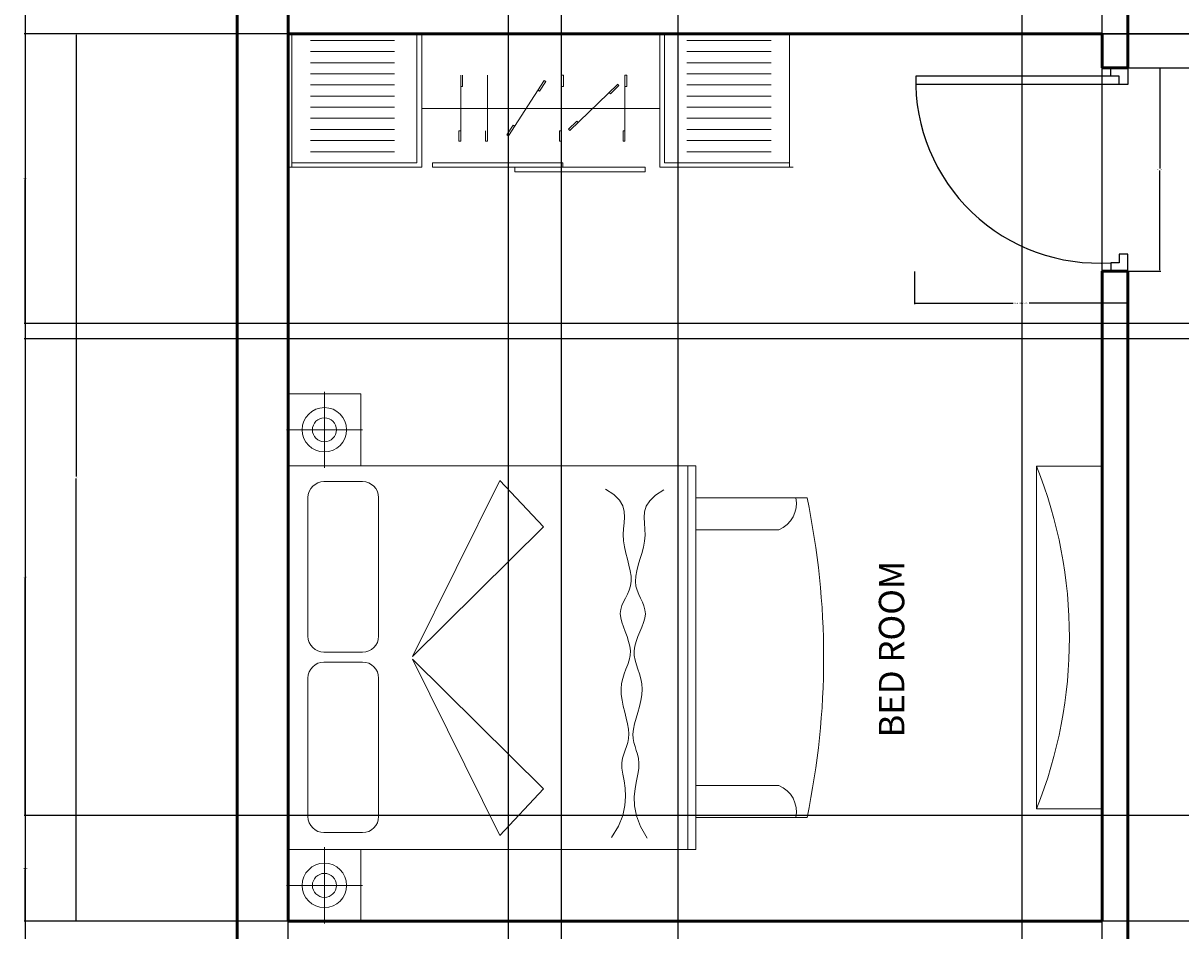
# Model space of a CAD drawing. Units: inches. Extents: x 1865 to 2541, y 1997 to 2759.
# Tile 6 of 11: x 1865 to 2070, y 2405 to 2566. Entities that reach past the tile are written whole.
import ezdxf

# ---------------------------------------------------------------- set-up
doc = ezdxf.new("R2010")
doc.units = ezdxf.units.IN
for name, color, linetype, lineweight in [('A-ANNO-DIMS', 2, 'Continuous', 18), ('A-AREA-IDEN', 4, 'Continuous', 18), ('A-WALL', 7, 'Continuous', 50), ('BED', 42, 'Continuous', 13), ('CUPBOARD', 61, 'Continuous', 18), ('DOOR', 1, 'Continuous', 25), ('TV', 3, 'Continuous', 18)]:
    doc.layers.add(name, color=color, linetype=linetype, lineweight=lineweight)
doc.styles.get("Standard").update_dxf_attribs({"font": 'arial.ttf'})
doc.dimstyles.get("Standard").update_dxf_attribs({"dimtxt": 0.18, "dimasz": 0.18, "dimexe": 0.18, "dimexo": 0.0625, "dimgap": 0.09, "dimtad": 0, "dimtih": 1, "dimtoh": 1, "dimdec": 4, "dimzin": 0, "dimdsep": 46, "dimtxsty": 'Standard', "dimcen": 0.09, "dimadec": 0, "dimazin": 0, "dimtfac": 1, "dimtdec": 4, "dimtofl": 0, "dimtmove": 0, "dimatfit": 3, "dimfxl": 1, "dimtolj": 1, "dimtzin": 0, "dimarcsym": 0})

# ---------------------------------------------------------------- blocks, each defined once
blk = doc.blocks.new('A$C4F543DC7')
for p, q in [((0.0134, 3.35, -0.1688), (3.3134, 3.35, -0.1688)), ((0.4634, 3.35, -0.1688), (0.0134, 3.35, -0.1688)), ((0.0134, 2.896, -0.1688), (0.0134, 3.35, -0.1688)), ((0.0134, 3.35, -0.1688), (0.0134, 2.896, -0.1688)), ((0.2381, 3.1233, -0.4388), (0.2381, 3.3614, -0.4388)), ((0.4634, 3.35, -0.1688), (0.4634, 0.8, -0.1688)), ((2.8634, 3.35, -0.1688), (0.4634, 3.35, -0.1688)), ((0.4634, 2.896, -0.1688), (0.4634, 3.35, -0.1688)), ((2.8634, 0.8, -0.1688), (2.8634, 3.35, -0.1688)), ((2.8634, 3.35, -0.1688), (3.3134, 3.35, -0.1688)), ((2.8634, 2.896, -0.1688), (2.8634, 3.35, -0.1688)), ((3.0888, 3.1233, -0.4388), (3.0888, 3.3614, -0.4388)), ((3.3134, 3.35, -0.1688), (3.3134, 2.896, -0.1688)), ((3.3134, 3.35, -0.1688), (3.3134, 2.896, -0.1688)), ((1.5354, 3.226, -0.1688), (0.6684, 3.226, -0.1688)), ((2.6644, 3.226, -0.1688), (1.7974, 3.226, -0.1688)), ((0.2381, 3.1233, -0.4388), (0, 3.1233, -0.4388)), ((0.2381, 3.1233, -0.4388), (0.4762, 3.1233, -0.4388)), ((0.2381, 3.1233, -0.4388), (0.2381, 2.8852, -0.4388)), ((0.5684, 3.126, -0.1688), (0.5684, 2.884, -0.1688)), ((1.6354, 2.884, -0.1688), (1.6354, 3.126, -0.1688)), ((1.6974, 3.126, -0.1688), (1.6974, 2.884, -0.1688)), ((2.7644, 2.884, -0.1688), (2.7644, 3.126, -0.1688)), ((3.0888, 3.1233, -0.4388), (2.8507, 3.1233, -0.4388)), ((3.0888, 3.1233, -0.4388), (3.0888, 2.8852, -0.4388)), ((3.0888, 3.1233, -0.4388), (3.3269, 3.1233, -0.4388)), ((0.4634, 2.896, -0.1688), (0.0134, 2.896, -0.1688)), ((0.0134, 2.896, -0.1688), (0.4634, 2.896, -0.1688)), ((0.4634, 0.8, -0.1688), (0.4634, 2.896, -0.1688)), ((2.8634, 2.896, -0.1688), (2.8634, 0.8, -0.1688)), ((3.3134, 2.896, -0.1688), (2.8634, 2.896, -0.1688)), ((3.3134, 2.896, -0.1688), (2.8634, 2.896, -0.1688)), ((0.6684, 2.784, -0.1688), (1.5354, 2.784, -0.1688)), ((1.7974, 2.784, -0.1688), (2.6644, 2.784, -0.1688)), ((1.6534, 2.573, -0.1688), (0.5504, 2.025, -0.1688)), ((0.8414, 1.752, -0.1688), (1.6534, 2.573, -0.1688)), ((2.4814, 1.752, -0.1688), (1.6694, 2.573, -0.1688)), ((1.6694, 2.573, -0.1688), (2.7724, 2.025, -0.1688)), ((0.5504, 2.025, -0.1688), (0.8414, 1.752, -0.1688)), ((2.7724, 2.025, -0.1688), (2.4814, 1.752, -0.1688)), ((0.5369, 1.3267, -0.1688), (0.6088, 1.2835, -0.1688)), ((2.6479, 1.2774, -0.1688), (2.683, 1.312, -0.1688)), ((2.683, 1.312, -0.1688), (2.7182, 1.3641, -0.1688)), ((0.6088, 1.2835, -0.1688), (0.6756, 1.2566, -0.1688)), ((0.6756, 1.2566, -0.1688), (0.7373, 1.2428, -0.1688)), ((0.7373, 1.2428, -0.1688), (0.794, 1.239, -0.1688)), ((0.794, 1.239, -0.1688), (0.8457, 1.242, -0.1688)), ((0.8457, 1.242, -0.1688), (0.8925, 1.2489, -0.1688)), ((0.8925, 1.2489, -0.1688), (0.9345, 1.2564, -0.1688)), ((0.9345, 1.2564, -0.1688), (0.9718, 1.2615, -0.1688)), ((0.9718, 1.2615, -0.1688), (1.0044, 1.2617, -0.1688)), ((1.0044, 1.2617, -0.1688), (1.0334, 1.2578, -0.1688)), ((1.0334, 1.2578, -0.1688), (1.0597, 1.2509, -0.1688)), ((1.0597, 1.2509, -0.1688), (1.0842, 1.2424, -0.1688)), ((1.0842, 1.2424, -0.1688), (1.1081, 1.2336, -0.1688)), ((1.1081, 1.2336, -0.1688), (1.1322, 1.2257, -0.1688)), ((1.2498, 1.2264, -0.1688), (1.2852, 1.2347, -0.1688)), ((1.2852, 1.2347, -0.1688), (1.3218, 1.2441, -0.1688)), ((1.3218, 1.2441, -0.1688), (1.3591, 1.2533, -0.1688)), ((1.3591, 1.2533, -0.1688), (1.3963, 1.2612, -0.1688)), ((1.3963, 1.2612, -0.1688), (1.4328, 1.2664, -0.1688)), ((1.4328, 1.2664, -0.1688), (1.4679, 1.2677, -0.1688)), ((1.4679, 1.2677, -0.1688), (1.501, 1.2643, -0.1688)), ((1.501, 1.2643, -0.1688), (1.5324, 1.257, -0.1688)), ((1.5324, 1.257, -0.1688), (1.5624, 1.2473, -0.1688)), ((1.5624, 1.2473, -0.1688), (1.5915, 1.2365, -0.1688)), ((1.5915, 1.2365, -0.1688), (1.6199, 1.2259, -0.1688)), ((1.7955, 1.2301, -0.1688), (1.8258, 1.2417, -0.1688)), ((1.8258, 1.2417, -0.1688), (1.8557, 1.2531, -0.1688)), ((1.8557, 1.2531, -0.1688), (1.8849, 1.263, -0.1688)), ((1.8849, 1.263, -0.1688), (1.913, 1.2698, -0.1688)), ((1.913, 1.2698, -0.1688), (1.9397, 1.2722, -0.1688)), ((1.9397, 1.2722, -0.1688), (1.9649, 1.2692, -0.1688)), ((1.9649, 1.2692, -0.1688), (1.989, 1.2617, -0.1688)), ((1.989, 1.2617, -0.1688), (2.0124, 1.2512, -0.1688)), ((2.0124, 1.2512, -0.1688), (2.0359, 1.2391, -0.1688)), ((2.0359, 1.2391, -0.1688), (2.0599, 1.2269, -0.1688)), ((2.2791, 1.2279, -0.1688), (2.3173, 1.2378, -0.1688)), ((2.3173, 1.2378, -0.1688), (2.3558, 1.2465, -0.1688)), ((2.3558, 1.2465, -0.1688), (2.3944, 1.2527, -0.1688)), ((2.3944, 1.2527, -0.1688), (2.4325, 1.255, -0.1688)), ((2.4325, 1.255, -0.1688), (2.4698, 1.2529, -0.1688)), ((2.4698, 1.2529, -0.1688), (2.5064, 1.2488, -0.1688)), ((2.5064, 1.2488, -0.1688), (2.5423, 1.2459, -0.1688)), ((2.5423, 1.2459, -0.1688), (2.5777, 1.2476, -0.1688)), ((2.5777, 1.2476, -0.1688), (2.6129, 1.257, -0.1688)), ((2.6129, 1.257, -0.1688), (2.6479, 1.2774, -0.1688)), ((0.6067, 1.1458, -0.1688), (0.6743, 1.1706, -0.1688)), ((0.6743, 1.1706, -0.1688), (0.7364, 1.1825, -0.1688)), ((0.7364, 1.1825, -0.1688), (0.7931, 1.1846, -0.1688)), ((0.7931, 1.1846, -0.1688), (0.8447, 1.1799, -0.1688)), ((0.8447, 1.1799, -0.1688), (0.8913, 1.1716, -0.1688)), ((0.8913, 1.1716, -0.1688), (0.9331, 1.1628, -0.1688)), ((0.9331, 1.1628, -0.1688), (0.9701, 1.1565, -0.1688)), ((1.0318, 1.1582, -0.1688), (1.0583, 1.1642, -0.1688)), ((1.0583, 1.1642, -0.1688), (1.0831, 1.172, -0.1688)), ((1.0831, 1.172, -0.1688), (1.1072, 1.18, -0.1688)), ((1.1072, 1.18, -0.1688), (1.1316, 1.1872, -0.1688)), ((1.1316, 1.1872, -0.1688), (1.1573, 1.192, -0.1688)), ((1.1322, 1.2257, -0.1688), (1.1577, 1.2201, -0.1688)), ((1.1573, 1.192, -0.1688), (1.1851, 1.1932, -0.1688)), ((1.1577, 1.2201, -0.1688), (1.1855, 1.218, -0.1688)), ((1.1851, 1.1932, -0.1688), (1.2158, 1.1898, -0.1688)), ((1.1855, 1.218, -0.1688), (1.2163, 1.2204, -0.1688)), ((1.2158, 1.1898, -0.1688), (1.2491, 1.1828, -0.1688)), ((1.2163, 1.2204, -0.1688), (1.2498, 1.2264, -0.1688)), ((1.2491, 1.1828, -0.1688), (1.2842, 1.1734, -0.1688)), ((1.2842, 1.1734, -0.1688), (1.3206, 1.1629, -0.1688)), ((1.3206, 1.1629, -0.1688), (1.3575, 1.1524, -0.1688)), ((1.5609, 1.152, -0.1688), (1.5903, 1.1619, -0.1688)), ((1.5903, 1.1619, -0.1688), (1.6191, 1.1716, -0.1688)), ((1.6191, 1.1716, -0.1688), (1.6475, 1.1797, -0.1688)), ((1.6199, 1.2259, -0.1688), (1.6481, 1.2169, -0.1688)), ((1.6475, 1.1797, -0.1688), (1.676, 1.1849, -0.1688)), ((1.6481, 1.2169, -0.1688), (1.6765, 1.2108, -0.1688)), ((1.676, 1.1849, -0.1688), (1.7049, 1.1858, -0.1688)), ((1.6765, 1.2108, -0.1688), (1.7053, 1.209, -0.1688)), ((1.7049, 1.1858, -0.1688), (1.7344, 1.1816, -0.1688)), ((1.7053, 1.209, -0.1688), (1.7349, 1.2124, -0.1688)), ((1.7344, 1.1816, -0.1688), (1.7643, 1.1731, -0.1688)), ((1.7349, 1.2124, -0.1688), (1.7651, 1.2199, -0.1688)), ((1.7643, 1.1731, -0.1688), (1.7944, 1.1619, -0.1688)), ((1.7651, 1.2199, -0.1688), (1.7955, 1.2301, -0.1688)), ((1.7944, 1.1619, -0.1688), (1.8244, 1.1494, -0.1688)), ((2.0588, 1.1568, -0.1688), (2.0842, 1.167, -0.1688)), ((2.0599, 1.2269, -0.1688), (2.0849, 1.216, -0.1688)), ((2.0842, 1.167, -0.1688), (2.1112, 1.1743, -0.1688)), ((2.0849, 1.216, -0.1688), (2.1117, 1.2077, -0.1688)), ((2.1112, 1.1743, -0.1688), (2.1403, 1.1775, -0.1688)), ((2.1117, 1.2077, -0.1688), (2.1407, 1.2037, -0.1688)), ((2.1403, 1.1775, -0.1688), (2.1718, 1.1755, -0.1688)), ((2.1407, 1.2037, -0.1688), (2.1723, 1.2047, -0.1688)), ((2.1718, 1.1755, -0.1688), (2.2056, 1.1691, -0.1688)), ((2.1723, 1.2047, -0.1688), (2.2062, 1.21, -0.1688)), ((2.2056, 1.1691, -0.1688), (2.2411, 1.1598, -0.1688)), ((2.2062, 1.21, -0.1688), (2.242, 1.2182, -0.1688)), ((2.2411, 1.1598, -0.1688), (2.2779, 1.1489, -0.1688)), ((2.242, 1.2182, -0.1688), (2.2791, 1.2279, -0.1688)), ((0.5334, 1.105, -0.1688), (0.6067, 1.1458, -0.1688)), ((0.9701, 1.1565, -0.1688), (1.0027, 1.1552, -0.1688)), ((1.0027, 1.1552, -0.1688), (1.0318, 1.1582, -0.1688)), ((1.3575, 1.1524, -0.1688), (1.3945, 1.1434, -0.1688)), ((1.3945, 1.1434, -0.1688), (1.4308, 1.1371, -0.1688)), ((1.4308, 1.1371, -0.1688), (1.4658, 1.1347, -0.1688)), ((1.4658, 1.1347, -0.1688), (1.499, 1.137, -0.1688)), ((1.499, 1.137, -0.1688), (1.5306, 1.1433, -0.1688)), ((1.5306, 1.1433, -0.1688), (1.5609, 1.152, -0.1688)), ((1.8244, 1.1494, -0.1688), (1.8539, 1.137, -0.1688)), ((1.8539, 1.137, -0.1688), (1.8827, 1.1263, -0.1688)), ((1.8827, 1.1263, -0.1688), (1.9106, 1.1186, -0.1688)), ((1.9106, 1.1186, -0.1688), (1.9373, 1.1153, -0.1688)), ((1.9373, 1.1153, -0.1688), (1.9625, 1.1176, -0.1688)), ((1.9625, 1.1176, -0.1688), (1.9868, 1.1243, -0.1688)), ((1.9868, 1.1243, -0.1688), (2.0106, 1.134, -0.1688)), ((2.0106, 1.134, -0.1688), (2.0344, 1.1454, -0.1688)), ((2.0344, 1.1454, -0.1688), (2.0588, 1.1568, -0.1688)), ((2.2779, 1.1489, -0.1688), (2.3157, 1.1379, -0.1688)), ((2.3157, 1.1379, -0.1688), (2.354, 1.1279, -0.1688)), ((2.354, 1.1279, -0.1688), (2.3923, 1.1205, -0.1688)), ((2.3923, 1.1205, -0.1688), (2.4304, 1.117, -0.1688)), ((2.4304, 1.117, -0.1688), (2.4677, 1.118, -0.1688)), ((2.4677, 1.118, -0.1688), (2.5043, 1.1209, -0.1688)), ((2.5043, 1.1209, -0.1688), (2.5403, 1.1226, -0.1688)), ((2.5403, 1.1226, -0.1688), (2.5757, 1.1199, -0.1688)), ((2.5757, 1.1199, -0.1688), (2.6106, 1.1094, -0.1688)), ((2.6106, 1.1094, -0.1688), (2.645, 1.0879, -0.1688)), ((2.645, 1.0879, -0.1688), (2.6789, 1.0522, -0.1688)), ((2.6789, 1.0522, -0.1688), (2.7124, 0.999, -0.1688)), ((0.4634, 0.85, -0.1688), (2.8634, 0.85, -0.1688)), ((0.4634, 0.8, -0.1688), (2.8634, 0.8, -0.1688)), ((0.6634, 0.8, -0.1688), (0.4634, 0.8, -0.1688)), ((0.6634, 0.8, -0.1688), (2.6634, 0.8, -0.1688)), ((0.6634, 0.104, -0.1688), (0.6634, 0.8, -0.1688)), ((0.6634, 0.104, -0.1688), (0.6634, 0.8, -0.1688)), ((0.8634, 0.281, -0.1688), (0.8634, 0.8, -0.1688)), ((2.4634, 0.8, -0.1688), (2.4634, 0.281, -0.1688)), ((2.8634, 0.8, -0.1688), (2.6634, 0.8, -0.1688)), ((2.6634, 0.8, -0.1688), (2.6634, 0.104, -0.1688)), ((2.6634, 0.8, -0.1688), (2.6634, 0.104, -0.1688))]:
    blk.add_line(p, q)
for centre, radius in [((0.2381, 3.1233, -0.4388), 0.139), ((3.0888, 3.1233, -0.4388), 0.139), ((0.2381, 3.1233, -0.4388), 0.075), ((3.0888, 3.1233, -0.4388), 0.075)]:
    blk.add_circle(centre, radius)
for centre, radius, start, end in [((0.6684, 3.126, -0.1688), 0.1, 90, 180), ((1.5354, 3.126, -0.1688), 0.1, 0, 90), ((1.7974, 3.126, -0.1688), 0.1, 90, 180), ((2.6644, 3.126, -0.1688), 0.1, 0, 90), ((0.6684, 2.884, -0.1688), 0.1, 180, 270), ((1.5354, 2.884, -0.1688), 0.1, 270, 0), ((1.7974, 2.884, -0.1688), 0.1, 180, 270), ((2.6644, 2.884, -0.1688), 0.1, 270, 0), ((0.6994, 0.3472, -0.1688), 0.1769, 258.2616, 338.03196), ((2.6275, 0.3472, -0.1688), 0.1769, 201.96804, 281.7384), ((1.6634, 4.8597, -0.1688), 4.8597, 258.12517, 281.87483), ((1.6634, 4.8597, -0.1688), 4.8597, 258.12517, 281.87483)]:
    blk.add_arc(centre, radius, start, end)
blk = doc.blocks.new('A$C34930FF8')
at = {"ltscale": 0.05}
for p, q in [((0, 2252.4), (0, 16.8)), ((600, 2252.4), (0, 2252.4)), ((185.4, 1513), (185.4, 1521.5)), ((237.7, 1513), (237.7, 1521.5)), ((436.7, 1513), (436.7, 1504.4)), ((482.5, 1513), (482.5, 1504.4)), ((227.1, 1479.2), (233.2, 1485.2)), ((263.6, 1441.7), (269.7, 1447.7)), ((398.2, 1303.6), (392.1, 1297.6)), ((434.8, 1266.1), (428.7, 1260.1)), ((185.4, 1229.1), (185.4, 1237.7)), ((237.7, 1229.1), (237.7, 1237.7)), ((436.7, 1228.2), (436.7, 1219.7)), ((482.5, 1228.2), (482.5, 1219.7)), ((209.5, 1150.1), (214.1, 1157.3)), ((253.5, 1121.8), (258.1, 1129)), ((415.3, 1017.6), (410.6, 1010.5)), ((459.3, 989.3), (454.7, 982.1)), ((482.5, 894.9), (482.5, 886.3)), ((237.7, 775.3), (237.7, 783.9)), ((436.7, 775.3), (436.7, 766.8)), ((482.5, 775.3), (482.5, 766.8)), ((600, 16.8), (0, 16.8))]:
    blk.add_line(p, q, dxfattribs=at)
for p, q in [((580, 1690.9), (580, 2252.4)), ((600, 1669.3), (600, 2269.3)), ((30, 1790.9), (30, 2169.3)), ((80, 1790.9), (80, 2169.3)), ((130, 1790.9), (130, 2169.3)), ((180, 1790.9), (180, 2169.3)), ((230, 1790.9), (230, 2169.3)), ((280, 1790.9), (280, 2169.3)), ((330, 1790.9), (330, 2169.3)), ((380, 1790.9), (380, 2169.3)), ((430, 1790.9), (430, 2169.3)), ((480, 1790.9), (480, 2169.3)), ((530, 1790.9), (530, 2169.3)), ((580, 1690.9), (0, 1690.9)), ((600, 1669.3), (0, 1669.3)), ((335.4, 1666.1), (335.4, 603.1)), ((600, 1603.3), (620, 1603.3)), ((600, 1018.7), (600, 1603.3)), ((620, 1603.3), (620, 1018.7)), ((237.7, 1521.5), (185.4, 1521.5)), ((482.5, 1513), (185.4, 1513)), ((434.8, 1266.1), (227.4, 1478.9)), ((269.7, 1447.7), (233.2, 1485.2)), ((436.7, 1504.4), (482.5, 1504.4)), ((428.7, 1260.1), (392.1, 1297.6)), ((237.7, 1237.7), (185.4, 1237.7)), ((482.5, 1228.2), (185.4, 1228.2)), ((436.7, 1219.7), (482.5, 1219.7)), ((600, 1233.4), (580, 1233.4)), ((580, 1233.4), (580, 648.7)), ((600, 648.7), (600, 1233.4)), ((459.3, 989.3), (209.5, 1150.1)), ((258.1, 1129), (214.1, 1157.3)), ((454.7, 982.1), (410.6, 1010.5)), ((620, 1018.7), (600, 1018.7)), ((482.5, 894.9), (185.4, 894.9)), ((436.7, 886.3), (482.5, 886.3)), ((237.7, 783.9), (185.4, 783.9)), ((482.5, 775.3), (185.4, 775.3)), ((436.7, 766.8), (482.5, 766.8)), ((580, 648.7), (600, 648.7)), ((600, 600), (0, 600)), ((580, 578.3), (0, 578.3)), ((580, 578.3), (580, 16.8)), ((600, 600), (600, 0)), ((30, 478.3), (30, 100)), ((80, 478.3), (80, 100)), ((130, 478.3), (130, 100)), ((180, 478.3), (180, 100)), ((230, 478.3), (230, 100)), ((280, 478.3), (280, 100)), ((330, 478.3), (330, 100)), ((380, 478.3), (380, 100)), ((430, 478.3), (430, 100)), ((480, 478.3), (480, 100)), ((530, 478.3), (530, 100))]:
    blk.add_line(p, q)
blk = doc.blocks.new('DOOR-SWING-36IN')
for p, q in [((34.51, 36), (37.51, 36)), ((34.51, 34.5), (34.51, 36)), ((37.51, 36), (37.51, 33)), ((36.01, 34.5), (0.01, 34.5)), ((36.01, 33), (0.01, 33)), ((36.01, 34.5), (34.51, 34.5)), ((36.01, 33), (36.01, 34.5)), ((37.51, 33), (36.01, 33)), ((37.51, 3), (36.01, 3)), ((36.01, 3), (36.01, 1.5)), ((37.51, 0), (37.51, 3)), ((36.01, 1.5), (34.51, 1.5)), ((34.51, 1.5), (34.51, 0)), ((34.51, 0), (37.51, 0))]:
    blk.add_line(p, q)
blk.add_arc((32.32, 33.75), 32.32, 178.6705, 273.8756)
blk = doc.blocks.new('TV-UNIT')
blk.add_lwpolyline([(0, 11.62), (60.65, 11.62), (60.65, 0), (0, 0)], close=True)
blk.add_arc((30.32, -76.26), 82.06, 68.3146, 111.6854)
blk = doc.blocks.new('*D20')
at = {"layer": 'A-ANNO-DIMS', "color": 0, "lineweight": -2, "transparency": 16777216}
for p, q in [((2023.03, 2521.89), (2023.03, 2516.11)), ((2060.74, 2521.89), (2060.74, 2516.11)), ((2023.21, 2516.29), (2040.49, 2516.29)), ((2060.56, 2516.29), (2043.28, 2516.29))]:
    blk.add_line(p, q, dxfattribs=at)
at = {"layer": 'A-ANNO-DIMS', "color": 0, "transparency": 16777216}
for points in [[(2023.21, 2516.32), (2023.21, 2516.26), (2023.03, 2516.29)], [(2060.56, 2516.32), (2060.56, 2516.26), (2060.74, 2516.29)]]:
    blk.add_solid(points, dxfattribs=at)
at = {"layer": 'Defpoints', "color": 0, "transparency": 16777216}
for p in [(2023.03, 2521.95), (2060.74, 2521.95), (2060.74, 2516.29)]:
    blk.add_point(p, dxfattribs=at)
at = {"layer": 'A-ANNO-DIMS', "color": 0, "transparency": 16777216, "insert": (2041.89, 2516.29), "char_height": 0.18, "attachment_point": 5}
blk.add_mtext('\\A1;DOOR SWING 38 TYP.', dxfattribs=at)
blk = doc.blocks.new('*D21')
at = {"layer": 'A-ANNO-DIMS', "color": 0, "lineweight": -2, "transparency": 16777216}
for p, q in [((2060.81, 2557.95), (2066.58, 2557.95)), ((2066.4, 2557.77), (2066.4, 2540.13)), ((2066.4, 2522.13), (2066.4, 2539.77)), ((2060.81, 2521.95), (2066.58, 2521.95))]:
    blk.add_line(p, q, dxfattribs=at)
at = {"layer": 'A-ANNO-DIMS', "color": 0, "transparency": 16777216}
for points in [[(2066.37, 2557.77), (2066.43, 2557.77), (2066.4, 2557.95)], [(2066.37, 2522.13), (2066.43, 2522.13), (2066.4, 2521.95)]]:
    blk.add_solid(points, dxfattribs=at)
at = {"layer": 'Defpoints', "color": 0, "transparency": 16777216}
for p in [(2060.74, 2557.95), (2066.4, 2557.95), (2060.74, 2521.95)]:
    blk.add_point(p, dxfattribs=at)
at = {"layer": 'A-ANNO-DIMS', "color": 0, "transparency": 16777216, "insert": (2066.4, 2539.95), "char_height": 0.18, "attachment_point": 5}
blk.add_mtext('\\A1;36 TYP.', dxfattribs=at)
blk = doc.blocks.new('*D42')
at = {"layer": 'A-ANNO-DIMS', "color": 0, "lineweight": -2, "transparency": 16777216}
for p, q in [((1903.18, 2721.45), (1865.56, 2721.45)), ((1865.74, 2721.27), (1865.74, 2391.63)), ((1865.74, 2061.63), (1865.74, 2391.27)), ((1903.18, 2061.45), (1865.56, 2061.45))]:
    blk.add_line(p, q, dxfattribs=at)
at = {"layer": 'A-ANNO-DIMS', "color": 0, "transparency": 16777216}
for points in [[(1865.71, 2721.27), (1865.77, 2721.27), (1865.74, 2721.45)], [(1865.71, 2061.63), (1865.77, 2061.63), (1865.74, 2061.45)]]:
    blk.add_solid(points, dxfattribs=at)
at = {"layer": 'Defpoints', "color": 0, "transparency": 16777216}
for p in [(1865.74, 2721.45), (1903.24, 2721.45), (1903.24, 2061.45)]:
    blk.add_point(p, dxfattribs=at)
at = {"layer": 'A-ANNO-DIMS', "color": 0, "transparency": 16777216, "insert": (1865.74, 2391.45), "char_height": 0.18, "attachment_point": 5}
blk.add_mtext('\\A1;660', dxfattribs=at)
blk = doc.blocks.new('*D48')
at = {"layer": 'A-ANNO-DIMS', "color": 0, "lineweight": -2, "transparency": 16777216}
for p, q in [((1912.18, 2563.95), (1874.56, 2563.95)), ((1874.74, 2563.77), (1874.74, 2485.63)), ((1874.74, 2407.13), (1874.74, 2485.27)), ((1912.18, 2406.95), (1874.56, 2406.95))]:
    blk.add_line(p, q, dxfattribs=at)
at = {"layer": 'A-ANNO-DIMS', "color": 0, "transparency": 16777216}
for points in [[(1874.71, 2563.77), (1874.77, 2563.77), (1874.74, 2563.95)], [(1874.71, 2407.13), (1874.77, 2407.13), (1874.74, 2406.95)]]:
    blk.add_solid(points, dxfattribs=at)
at = {"layer": 'Defpoints', "color": 0, "transparency": 16777216}
for p in [(1874.74, 2563.95), (1912.24, 2563.95), (1912.24, 2406.95)]:
    blk.add_point(p, dxfattribs=at)
at = {"layer": 'A-ANNO-DIMS', "color": 0, "transparency": 16777216, "insert": (1874.74, 2485.45), "char_height": 0.18, "attachment_point": 5}
blk.add_mtext('\\A1;157', dxfattribs=at)
blk = doc.blocks.new('*D63')
at = {"layer": 'A-ANNO-DIMS', "color": 0, "lineweight": -2, "transparency": 16777216}
for p, q in [((2404.18, 2563.95), (1865.56, 2563.95)), ((1865.74, 2563.77), (1865.74, 2538.51)), ((1865.74, 2512.9), (1865.74, 2538.15)), ((2404.18, 2512.72), (1865.56, 2512.72))]:
    blk.add_line(p, q, dxfattribs=at)
at = {"layer": 'A-ANNO-DIMS', "color": 0, "transparency": 16777216}
for points in [[(1865.71, 2563.77), (1865.77, 2563.77), (1865.74, 2563.95)], [(1865.71, 2512.9), (1865.77, 2512.9), (1865.74, 2512.72)]]:
    blk.add_solid(points, dxfattribs=at)
at = {"layer": 'Defpoints', "color": 0, "transparency": 16777216}
for p in [(2404.24, 2563.95), (1865.74, 2512.72), (2404.24, 2512.72)]:
    blk.add_point(p, dxfattribs=at)
at = {"layer": 'A-ANNO-DIMS', "color": 0, "transparency": 16777216, "insert": (1865.74, 2538.33), "char_height": 0.18, "attachment_point": 5}
blk.add_mtext('\\A1;51.23', dxfattribs=at)
blk = doc.blocks.new('*D66')
at = {"layer": 'A-ANNO-DIMS', "color": 0, "lineweight": -2, "transparency": 16777216}
for p, q in [((2408.32, 2425.66), (1865.56, 2425.66)), ((1865.74, 2425.48), (1865.74, 2416.48)), ((1865.74, 2407.13), (1865.74, 2416.12)), ((2408.32, 2406.95), (1865.56, 2406.95))]:
    blk.add_line(p, q, dxfattribs=at)
at = {"layer": 'A-ANNO-DIMS', "color": 0, "transparency": 16777216}
for points in [[(1865.71, 2425.48), (1865.77, 2425.48), (1865.74, 2425.66)], [(1865.71, 2407.13), (1865.77, 2407.13), (1865.74, 2406.95)]]:
    blk.add_solid(points, dxfattribs=at)
at = {"layer": 'Defpoints', "color": 0, "transparency": 16777216}
for p in [(2408.38, 2425.66), (1865.74, 2406.95), (2408.38, 2406.95)]:
    blk.add_point(p, dxfattribs=at)
at = {"layer": 'A-ANNO-DIMS', "color": 0, "transparency": 16777216, "insert": (1865.74, 2416.3), "char_height": 0.18, "attachment_point": 5}
blk.add_mtext('\\A1;18.706', dxfattribs=at)
blk = doc.blocks.new('*D67')
at = {"layer": 'A-ANNO-DIMS', "color": 0, "lineweight": -2, "transparency": 16777216}
for p, q in [((2475.89, 2509.99), (1865.56, 2509.99)), ((1865.74, 2509.81), (1865.74, 2468)), ((1865.74, 2425.84), (1865.74, 2467.64)), ((2475.89, 2425.66), (1865.56, 2425.66))]:
    blk.add_line(p, q, dxfattribs=at)
at = {"layer": 'A-ANNO-DIMS', "color": 0, "transparency": 16777216}
for points in [[(1865.71, 2509.81), (1865.77, 2509.81), (1865.74, 2509.99)], [(1865.71, 2425.84), (1865.77, 2425.84), (1865.74, 2425.66)]]:
    blk.add_solid(points, dxfattribs=at)
at = {"layer": 'Defpoints', "color": 0, "transparency": 16777216}
for p in [(1865.74, 2509.99), (2475.95, 2509.99), (2475.95, 2425.66)]:
    blk.add_point(p, dxfattribs=at)
at = {"layer": 'A-ANNO-DIMS', "color": 0, "transparency": 16777216, "insert": (1865.74, 2467.82), "char_height": 0.18, "attachment_point": 5}
blk.add_mtext('\\A1;84.33', dxfattribs=at)
blk = doc.blocks.new('*D68')
at = {"layer": 'A-ANNO-DIMS', "color": 0, "lineweight": -2, "transparency": 16777216}
for p, q in [((1912.24, 2169.51), (1912.24, 2759.13)), ((1912.42, 2758.95), (1931.52, 2758.95)), ((1951.06, 2758.95), (1931.96, 2758.95)), ((1951.24, 2169.51), (1951.24, 2759.13))]:
    blk.add_line(p, q, dxfattribs=at)
at = {"layer": 'A-ANNO-DIMS', "color": 0, "transparency": 16777216}
for points in [[(1912.42, 2758.98), (1912.42, 2758.92), (1912.24, 2758.95)], [(1951.06, 2758.98), (1951.06, 2758.92), (1951.24, 2758.95)]]:
    blk.add_solid(points, dxfattribs=at)
at = {"layer": 'Defpoints', "color": 0, "transparency": 16777216}
for p in [(1951.24, 2758.95), (1912.24, 2169.45), (1951.24, 2169.45)]:
    blk.add_point(p, dxfattribs=at)
at = {"layer": 'A-ANNO-DIMS', "color": 0, "transparency": 16777216, "insert": (1931.74, 2758.95), "char_height": 0.18, "attachment_point": 5}
blk.add_mtext('\\A1;39', dxfattribs=at)
blk = doc.blocks.new('*D79')
at = {"layer": 'A-ANNO-DIMS', "color": 0, "lineweight": -2, "transparency": 16777216}
for p, q in [((2056.31, 2563.95), (2093.92, 2563.95)), ((2093.74, 2563.77), (2093.74, 2561.13)), ((2093.74, 2558.13), (2093.74, 2560.77)), ((2056.31, 2557.95), (2093.92, 2557.95))]:
    blk.add_line(p, q, dxfattribs=at)
at = {"layer": 'A-ANNO-DIMS', "color": 0, "transparency": 16777216}
for points in [[(2093.71, 2563.77), (2093.77, 2563.77), (2093.74, 2563.95)], [(2093.71, 2558.13), (2093.77, 2558.13), (2093.74, 2557.95)]]:
    blk.add_solid(points, dxfattribs=at)
at = {"layer": 'Defpoints', "color": 0, "transparency": 16777216}
for p in [(2056.24, 2563.95), (2056.24, 2557.95), (2093.74, 2557.95)]:
    blk.add_point(p, dxfattribs=at)
at = {"layer": 'A-ANNO-DIMS', "color": 0, "transparency": 16777216, "insert": (2093.74, 2560.95), "char_height": 0.18, "attachment_point": 5}
blk.add_mtext('\\A1;6', dxfattribs=at)
blk = doc.blocks.new('*D81')
at = {"layer": 'A-ANNO-DIMS', "color": 0, "lineweight": -2, "transparency": 16777216}
for p, q in [((1960.58, 2070.51), (1960.58, 2759.13)), ((1960.76, 2758.95), (1970.44, 2758.95)), ((1981.06, 2758.95), (1971.38, 2758.95)), ((1981.24, 2070.51), (1981.24, 2759.13))]:
    blk.add_line(p, q, dxfattribs=at)
at = {"layer": 'A-ANNO-DIMS', "color": 0, "transparency": 16777216}
for points in [[(1960.76, 2758.98), (1960.76, 2758.92), (1960.58, 2758.95)], [(1981.06, 2758.98), (1981.06, 2758.92), (1981.24, 2758.95)]]:
    blk.add_solid(points, dxfattribs=at)
at = {"layer": 'Defpoints', "color": 0, "transparency": 16777216}
for p in [(1960.58, 2758.95), (1960.58, 2070.45), (1981.24, 2070.45)]:
    blk.add_point(p, dxfattribs=at)
at = {"layer": 'A-ANNO-DIMS', "color": 0, "transparency": 16777216, "insert": (1970.91, 2758.95), "char_height": 0.18, "attachment_point": 5}
blk.add_mtext('\\A1;20.665', dxfattribs=at)
blk = doc.blocks.new('*D82')
at = {"layer": 'A-ANNO-DIMS', "color": 0, "lineweight": -2, "transparency": 16777216}
for p, q in [((2042.07, 2070.51), (2042.07, 2759.13)), ((2042.25, 2758.95), (2048.7, 2758.95)), ((2056.06, 2758.95), (2049.61, 2758.95)), ((2056.24, 2070.51), (2056.24, 2759.13))]:
    blk.add_line(p, q, dxfattribs=at)
at = {"layer": 'A-ANNO-DIMS', "color": 0, "transparency": 16777216}
for points in [[(2042.25, 2758.98), (2042.25, 2758.92), (2042.07, 2758.95)], [(2056.06, 2758.98), (2056.06, 2758.92), (2056.24, 2758.95)]]:
    blk.add_solid(points, dxfattribs=at)
at = {"layer": 'Defpoints', "color": 0, "transparency": 16777216}
for p in [(2042.07, 2758.95), (2042.07, 2070.45), (2056.24, 2070.45)]:
    blk.add_point(p, dxfattribs=at)
at = {"layer": 'A-ANNO-DIMS', "color": 0, "transparency": 16777216, "insert": (2049.16, 2758.95), "char_height": 0.18, "attachment_point": 5}
blk.add_mtext('\\A1;14.176', dxfattribs=at)

msp = doc.modelspace()

# ---------------------------------------------------------------- linework, layer by layer
at = {"layer": 'A-WALL'}
for p, q in [((1903.243, 2721.4494), (1903.243, 2061.4494)), ((1912.243, 2712.4494), (1912.243, 2406.9494)), ((2060.743, 2563.9494), (2060.743, 2568.4494)), ((2056.243, 2563.9494), (1912.243, 2563.9494)), ((2056.243, 2563.9494), (2056.243, 2557.9494)), ((2060.743, 2563.9494), (2060.743, 2557.9494)), ((2060.743, 2557.9494), (2056.243, 2557.9494)), ((2060.743, 2521.9494), (2056.243, 2521.9494)), ((2056.243, 2521.9494), (2056.243, 2406.9494)), ((2060.743, 2521.9494), (2060.743, 2402.4494)), ((2056.243, 2406.9494), (1912.243, 2406.9494))]:
    msp.add_line(p, q, dxfattribs=at)

# ---------------------------------------------------------------- block references
at = {"layer": 'BED', "xscale": 28.27205529407425, "yscale": 28.27205529407425, "zscale": 28.27205529407425, "rotation": 90}
msp.add_blockref('A$C4F543DC7', (2006.9544, 2406.5695, 4.7709), dxfattribs=at)
at = {"layer": 'CUPBOARD', "xscale": 0.0393700787401575, "yscale": 0.0393700787401575, "zscale": 0.0393700787401575, "rotation": 270}
msp.add_blockref('A$C34930FF8', (1912.243, 2563.9494), dxfattribs=at)
at = {"layer": 'DOOR'}
msp.add_blockref('DOOR-SWING-36IN', (2023.234, 2521.949), dxfattribs=at)
at = {"layer": 'TV', "extrusion": (0, 0, -1), "zscale": -1, "rotation": 89.99999999999955}
msp.add_blockref('TV-UNIT', (-2044.6276, 2426.8211), dxfattribs=at)

# ---------------------------------------------------------------- texts
at = {"layer": 'A-AREA-IDEN', "insert": (2016.7208, 2439.465), "char_height": 4.5, "attachment_point": 1, "rotation": 90}
msp.add_mtext_dynamic_manual_height_columns('BED ROOM', width=66.075761, gutter_width=12.5, heights=[0], dxfattribs=at)

# ---------------------------------------------------------------- dimensions: what is measured, and where the dimension line sits
at = {"layer": 'A-ANNO-DIMS'}
for base, p1, p2, override, picture, middle in [((1951.243, 2758.9494), (1912.243, 2169.4494), (1951.243, 2169.4494), {"dimdec": 0, "dimlfac": 1, "dimrnd": 0, "dimzin": 0, "dimdsep": 46, "dimlunit": 2}, '*D68', (1931.743, 2758.9494)), ((1960.57848, 2758.94943), (1981.243, 2070.44943), (1960.57848, 2070.44943), {"dimdec": 3, "dimlfac": 1, "dimrnd": 0, "dimzin": 0, "dimdsep": 46, "dimlunit": 2}, '*D81', (1970.91074, 2758.94943)), ((2042.0671, 2758.9494), (2056.243, 2070.4494), (2042.0671, 2070.4494), {"dimdec": 3, "dimlfac": 1, "dimrnd": 0, "dimzin": 0, "dimdsep": 46, "dimlunit": 2}, '*D82', (2049.1551, 2758.9494))]:
    dim = msp.add_linear_dim(base=base, p1=p1, p2=p2, dimstyle='Standard', override=override, dxfattribs=at)
    dim.commit()
    dim.dimension.update_dxf_attribs({"geometry": picture, "text_midpoint": middle})
for base, p1, p2, angle, override, picture, middle in [((1865.743, 2721.4494), (1903.243, 2061.4494), (1903.243, 2721.4494), 90, {"dimdec": 0, "dimlfac": 1, "dimrnd": 0, "dimzin": 0, "dimdsep": 46, "dimlunit": 2}, '*D42', (1865.743, 2391.4494)), ((1865.743, 2512.7166), (2404.243, 2563.9494), (2404.243, 2512.7166), 90, {"dimdec": 2, "dimlfac": 1, "dimrnd": 0, "dimzin": 0, "dimdsep": 46, "dimlunit": 2}, '*D63', (1865.743, 2538.333)), ((1874.743, 2563.9494), (1912.243, 2406.9494), (1912.243, 2563.9494), 90, {"dimdec": 0, "dimlfac": 1, "dimrnd": 0, "dimzin": 0, "dimdsep": 46, "dimlunit": 2}, '*D48', (1874.743, 2485.4494)), ((2093.743, 2557.9494), (2056.243, 2563.9494), (2056.243, 2557.9494), 270, {"dimdec": 0, "dimlfac": 1, "dimrnd": 0, "dimzin": 0, "dimdsep": 46, "dimlunit": 2}, '*D79', (2093.743, 2560.9494)), ((1865.743, 2509.9875), (2475.9518, 2425.6552), (2475.9518, 2509.9875), 90, {"dimdec": 2, "dimlfac": 1, "dimrnd": 0, "dimzin": 0, "dimdsep": 46, "dimlunit": 2}, '*D67', (1865.743, 2467.8214)), ((1865.743, 2406.9494), (2408.3779, 2425.6552), (2408.3779, 2406.9494), 90, {"dimdec": 3, "dimlfac": 1, "dimrnd": 0, "dimzin": 0, "dimdsep": 46, "dimlunit": 2}, '*D66', (1865.743, 2416.3023))]:
    dim = msp.add_linear_dim(base=base, p1=p1, p2=p2, angle=angle, dimstyle='Standard', override=override, dxfattribs=at)
    dim.commit()
    dim.dimension.update_dxf_attribs({"geometry": picture, "text_midpoint": middle})
dim = msp.add_linear_dim(base=(2066.3996, 2557.9494), p1=(2060.743, 2521.9494), p2=(2060.743, 2557.9494), angle=90, text='<> TYP.', dimstyle='Standard', override={"dimdec": 0, "dimlfac": 1, "dimrnd": 0, "dimzin": 0, "dimdsep": 46, "dimlunit": 2}, dxfattribs=at)
dim.commit()
dim.dimension.update_dxf_attribs({"geometry": '*D21', "text_midpoint": (2066.3996, 2539.9494)})
dim = msp.add_linear_dim(base=(2060.743, 2516.2928), p1=(2023.0323, 2521.9494), p2=(2060.743, 2521.9494), text='DOOR SWING <> TYP.', dimstyle='Standard', override={"dimdec": 0, "dimlfac": 1, "dimrnd": 0, "dimzin": 0, "dimdsep": 46, "dimlunit": 2}, dxfattribs=at)
dim.commit()
dim.dimension.update_dxf_attribs({"geometry": '*D20', "text_midpoint": (2041.8876, 2516.2928)})

doc.saveas('drawing.dxf')
